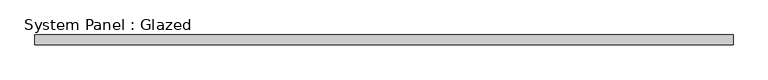
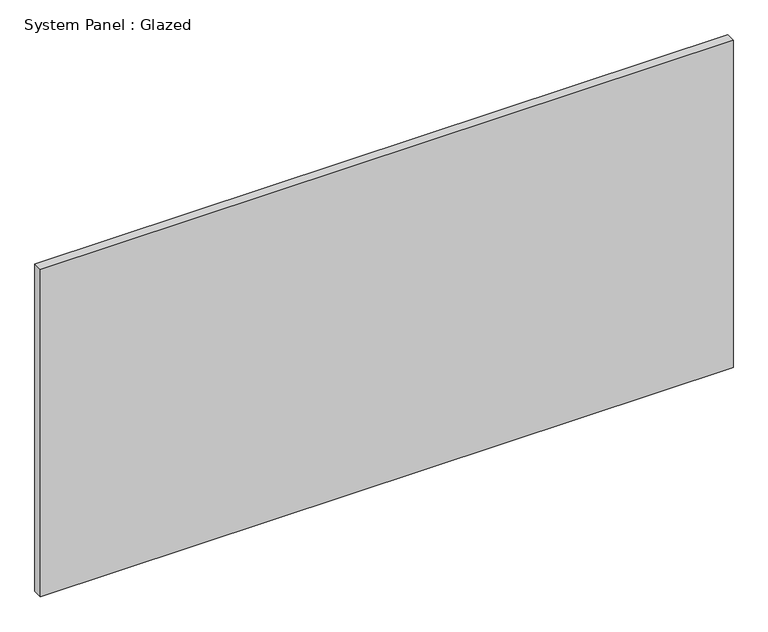
"""IFC4 building model written with IfcOpenShell, lengths in millimetres: plate geometry, System Panel : Glazed."""

from ifc_helpers import new_model, si_unit, origin, origin_with_axes, place, context, project, spatial, polyline, outline, extrude, source, transform, mapped, element, save


def system_panel_glazed_95be5de7(model_context):
    return source(origin(), model_context, "Body", "SweptSolid", [
        extrude(outline(polyline([(914.4, 19.05), (-914.4, 19.05), (-914.4, 44.45), (914.4, 44.45), (914.4, 19.05)])), origin_with_axes(), (0.0, 0.0, 1.0), 914.4),
    ])


if __name__ == "__main__":
    model = new_model("IFC4")
    model_context = context("Model", 3, world=origin())
    ifc_project = project(units=[si_unit("LENGTHUNIT", "METRE", prefix="MILLI")], contexts=[model_context])
    site = spatial("IfcSite", under=ifc_project)
    building = spatial("IfcBuilding", under=site)
    placement = place(None, origin())
    system_panel_glazed_shape = system_panel_glazed_95be5de7(model_context)
    element("IfcPlate", 1, ObjectType="System Panel : Glazed", at=placement, inside=building, context=model_context, shape_type="MappedRepresentation", body=[
        mapped(system_panel_glazed_shape, transform((0.0, 0.0, 0.0), x_axis=(1.0, 0.0, 0.0), y_axis=(0.0, 1.0, 0.0), z_axis=(0.0, 0.0, 1.0))),
    ])
    save(model, "model.ifc")

# Revit data of these elements
# Type "System Panel : Glazed"
#   Construction Type Id = "GSP4R"
#   Analytic Construction = "1/8 in Pilkington single glazing"
#   Visual Light Transmittance = 0.9
#   Solar Heat Gain Coefficient = 0.86
#   Heat Transfer Coefficient (U) = 6.7069 W/(m²·K)
# Element 1 (IfcPlate, "System Panel : Glazed")
#   Materials on its faces: "Glass"
# Materials
#   "Glass": class "Glass", colour RGB 0 128 192, transparency 0.75, Description = "Soda Lime Glass", Cost = 0
